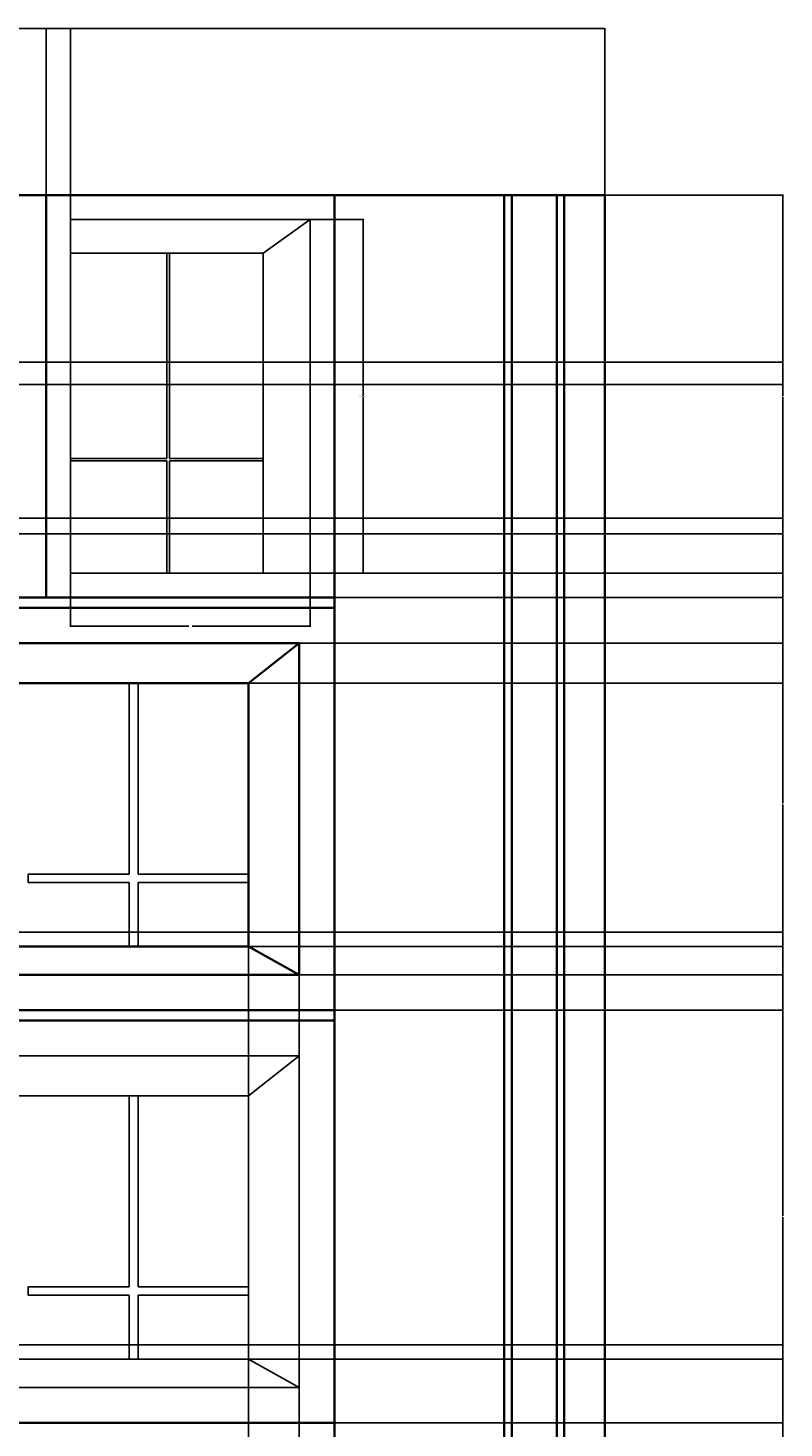
# Model space of a CAD drawing. Units: feet. Extents: x 1141 to 2858, y 751 to 1654.
# Tile 13 of 13: x 2610 to 2858, y 1195 to 1654. Entities that reach past the tile are written whole.
import ezdxf

# ---------------------------------------------------------------- set-up
doc = ezdxf.new("R2010")
doc.units = ezdxf.units.FT
for name, color, linetype, lineweight in [('A-ANNO-DIMS', 2, 'Continuous', 18), ('A-ELEV', 7, 'Continuous', 35), ('A-GLAZ', 4, 'Continuous', 25)]:
    doc.layers.add(name, color=color, linetype=linetype, lineweight=lineweight)
doc.styles.get("Standard").update_dxf_attribs({"font": 'arial.ttf'})
doc.dimstyles.get("Standard").update_dxf_attribs({"dimtxt": 0.18, "dimasz": 0.18, "dimexe": 0.18, "dimexo": 0.0625, "dimgap": 0.09, "dimtad": 0, "dimtih": 1, "dimtoh": 1, "dimdec": 1, "dimzin": 0, "dimdsep": 46, "dimlunit": 3, "dimtxsty": 'Standard', "dimcen": 0.09, "dimadec": 0, "dimazin": 0, "dimtfac": 1, "dimtdec": 1, "dimtofl": 0, "dimtmove": 0, "dimatfit": 3, "dimfxl": 1, "dimtolj": 1, "dimtzin": 0, "dimarcsym": 0})

# ---------------------------------------------------------------- blocks, each defined once
blk = doc.blocks.new('WIN-SIDE-B')
blk.add_line((63.09, 104.94), (78.57, 116.03))
blk.add_lwpolyline([(78.57, 0), (0, 0), (0, 116.03), (78.57, 116.03)], close=True)
for points in [[(63.09, 0), (63.09, 104.94), (0, 104.94)], [(31.54, 37.61), (31.54, 104.94), (32.46, 104.94), (32.46, 37.61)], [(31.54, 36.79), (0, 36.79), (0, 37.61), (31.54, 37.61)], [(32.46, 36.79), (32.46, 0), (31.54, 0), (31.54, 36.79)], [(32.46, 37.61), (63.09, 37.61), (63.09, 36.79), (32.46, 36.79)]]:
    blk.add_lwpolyline(points)
blk = doc.blocks.new('BALCONY-GLAZ-B')
for p, q in [((0, 108.84), (16.63, 95.74)), ((266.62, 95.74), (273.67, 108.84)), ((16.63, 95.74), (16.63, 9.29)), ((16.63, 95.74), (266.62, 95.74)), ((266.62, 95.74), (266.62, 9.19)), ((16.63, 9.29), (0, 0)), ((16.63, 9.29), (266.62, 9.29)), ((266.62, 9.29), (273.67, 0))]:
    blk.add_line(p, q)
for points in [[(0, 108.84), (273.67, 108.84), (273.67, 0), (0, 0)], [(266.62, 9.19), (168.47, 9.19), (168.47, 95.74), (266.62, 95.74)]]:
    blk.add_lwpolyline(points, close=True)
blk = doc.blocks.new('WIN-SLIDING')
for points in [[(36.16, 23.71), (36.16, 86.44), (39.2, 86.44), (39.2, 23.71)], [(36.16, 23.71), (0, 23.71), (0, 21.05), (36.16, 21.05)], [(39.2, 21.05), (72.32, 21.05), (72.32, 23.71), (39.2, 23.71)], [(39.2, 21.05), (39.2, 0), (36.16, 0), (36.16, 21.05)]]:
    blk.add_lwpolyline(points)
blk = doc.blocks.new('*D16')
at = {"layer": 'A-ANNO-DIMS', "color": 0, "lineweight": -2, "transparency": 16777216}
for p, q in [((2702.75, 1591.47), (2720.27, 1591.47)), ((2720.09, 1591.29), (2720.09, 1533.64)), ((2720.09, 1475.62), (2720.09, 1533.27)), ((2702.75, 1475.44), (2720.27, 1475.44))]:
    blk.add_line(p, q, dxfattribs=at)
at = {"layer": 'A-ANNO-DIMS', "color": 0, "transparency": 16777216}
for points in [[(2720.06, 1591.29), (2720.12, 1591.29), (2720.09, 1591.47)], [(2720.06, 1475.62), (2720.12, 1475.62), (2720.09, 1475.44)]]:
    blk.add_solid(points, dxfattribs=at)
at = {"layer": 'Defpoints', "color": 0, "transparency": 16777216}
for p in [(2702.69, 1591.47), (2720.09, 1591.47), (2702.69, 1475.44)]:
    blk.add_point(p, dxfattribs=at)
at = {"layer": 'A-ANNO-DIMS', "color": 0, "transparency": 16777216, "insert": (2720.09, 1533.45), "char_height": 0.18, "attachment_point": 5}
blk.add_mtext('\\A1;SIDE WINDOW B 116 TYP.', dxfattribs=at)
blk = doc.blocks.new('*D17')
at = {"layer": 'A-ANNO-DIMS', "color": 0, "lineweight": -2, "transparency": 16777216}
for p, q in [((2624.12, 1475.38), (2624.12, 1457.85)), ((2702.69, 1475.38), (2702.69, 1457.85)), ((2624.3, 1458.03), (2662.88, 1458.03)), ((2702.51, 1458.03), (2663.93, 1458.03))]:
    blk.add_line(p, q, dxfattribs=at)
at = {"layer": 'A-ANNO-DIMS', "color": 0, "transparency": 16777216}
for points in [[(2624.3, 1458.06), (2624.3, 1458), (2624.12, 1458.03)], [(2702.51, 1458.06), (2702.51, 1458), (2702.69, 1458.03)]]:
    blk.add_solid(points, dxfattribs=at)
at = {"layer": 'Defpoints', "color": 0, "transparency": 16777216}
for p in [(2624.12, 1475.44), (2702.69, 1475.44), (2702.69, 1458.03)]:
    blk.add_point(p, dxfattribs=at)
at = {"layer": 'A-ANNO-DIMS', "color": 0, "transparency": 16777216, "insert": (2663.41, 1458.03), "char_height": 0.18, "attachment_point": 5}
blk.add_mtext('\\A1;79 TYP.', dxfattribs=at)
blk = doc.blocks.new('*D31')
at = {"layer": 'A-ANNO-DIMS', "color": 0, "lineweight": -2, "transparency": 16777216}
for p, q in [((2117.47, 1196.68), (2857.83, 1196.68)), ((2857.65, 1196.5), (2857.65, 1129.16)), ((2857.65, 1061.47), (2857.65, 1128.8)), ((2117.47, 1061.29), (2857.83, 1061.29))]:
    blk.add_line(p, q, dxfattribs=at)
at = {"layer": 'A-ANNO-DIMS', "color": 0, "transparency": 16777216}
for points in [[(2857.62, 1196.5), (2857.68, 1196.5), (2857.65, 1196.68)], [(2857.62, 1061.47), (2857.68, 1061.47), (2857.65, 1061.29)]]:
    blk.add_solid(points, dxfattribs=at)
at = {"layer": 'Defpoints', "color": 0, "transparency": 16777216}
for p in [(2117.41, 1196.68), (2857.65, 1196.68), (2117.41, 1061.29)]:
    blk.add_point(p, dxfattribs=at)
at = {"layer": 'A-ANNO-DIMS', "color": 0, "transparency": 16777216, "insert": (2857.65, 1128.98), "char_height": 0.18, "attachment_point": 5}
blk.add_mtext('\\A1;135.4', dxfattribs=at)
blk = doc.blocks.new('*D32')
at = {"layer": 'A-ANNO-DIMS', "color": 0, "lineweight": -2, "transparency": 16777216}
for p, q in [((2117.47, 1332.06), (2857.83, 1332.06)), ((2857.65, 1331.88), (2857.65, 1264.55)), ((2857.65, 1196.86), (2857.65, 1264.19)), ((2117.47, 1196.68), (2857.83, 1196.68))]:
    blk.add_line(p, q, dxfattribs=at)
at = {"layer": 'A-ANNO-DIMS', "color": 0, "transparency": 16777216}
for points in [[(2857.62, 1331.88), (2857.68, 1331.88), (2857.65, 1332.06)], [(2857.62, 1196.86), (2857.68, 1196.86), (2857.65, 1196.68)]]:
    blk.add_solid(points, dxfattribs=at)
at = {"layer": 'Defpoints', "color": 0, "transparency": 16777216}
for p in [(2117.41, 1332.06), (2857.65, 1332.06), (2117.41, 1196.68)]:
    blk.add_point(p, dxfattribs=at)
at = {"layer": 'A-ANNO-DIMS', "color": 0, "transparency": 16777216, "insert": (2857.65, 1264.37), "char_height": 0.18, "attachment_point": 5}
blk.add_mtext('\\A1;135.4', dxfattribs=at)
blk = doc.blocks.new('*D33')
at = {"layer": 'A-ANNO-DIMS', "color": 0, "lineweight": -2, "transparency": 16777216}
for p, q in [((2117.47, 1467.45), (2857.83, 1467.45)), ((2857.65, 1467.27), (2857.65, 1399.94)), ((2857.65, 1332.24), (2857.65, 1399.58)), ((2117.47, 1332.06), (2857.83, 1332.06))]:
    blk.add_line(p, q, dxfattribs=at)
at = {"layer": 'A-ANNO-DIMS', "color": 0, "transparency": 16777216}
for points in [[(2857.62, 1467.27), (2857.68, 1467.27), (2857.65, 1467.45)], [(2857.62, 1332.24), (2857.68, 1332.24), (2857.65, 1332.06)]]:
    blk.add_solid(points, dxfattribs=at)
at = {"layer": 'Defpoints', "color": 0, "transparency": 16777216}
for p in [(2117.41, 1467.45), (2857.65, 1467.45), (2117.41, 1332.06)]:
    blk.add_point(p, dxfattribs=at)
at = {"layer": 'A-ANNO-DIMS', "color": 0, "transparency": 16777216, "insert": (2857.65, 1399.76), "char_height": 0.18, "attachment_point": 5}
blk.add_mtext('\\A1;135.4', dxfattribs=at)
blk = doc.blocks.new('*D34')
at = {"layer": 'A-ANNO-DIMS', "color": 0, "lineweight": -2, "transparency": 16777216}
for p, q in [((2117.47, 1599.45), (2857.83, 1599.45)), ((2857.65, 1599.27), (2857.65, 1533.63)), ((2857.65, 1467.63), (2857.65, 1533.27)), ((2117.47, 1467.45), (2857.83, 1467.45))]:
    blk.add_line(p, q, dxfattribs=at)
at = {"layer": 'A-ANNO-DIMS', "color": 0, "transparency": 16777216}
for points in [[(2857.62, 1599.27), (2857.68, 1599.27), (2857.65, 1599.45)], [(2857.62, 1467.63), (2857.68, 1467.63), (2857.65, 1467.45)]]:
    blk.add_solid(points, dxfattribs=at)
at = {"layer": 'Defpoints', "color": 0, "transparency": 16777216}
for p in [(2117.41, 1599.45), (2857.65, 1599.45), (2117.41, 1467.45)]:
    blk.add_point(p, dxfattribs=at)
at = {"layer": 'A-ANNO-DIMS', "color": 0, "transparency": 16777216, "insert": (2857.65, 1533.45), "char_height": 0.18, "attachment_point": 5}
blk.add_mtext('\\A1;132', dxfattribs=at)
blk = doc.blocks.new('*D35')
at = {"layer": 'A-ANNO-DIMS', "color": 0, "lineweight": -2, "transparency": 16777216}
for p, q in [((2319.3, 1599.52), (2319.3, 1654.28)), ((2319.48, 1654.1), (2559.01, 1654.1)), ((2799.12, 1654.1), (2559.59, 1654.1)), ((2799.3, 1599.52), (2799.3, 1654.28))]:
    blk.add_line(p, q, dxfattribs=at)
at = {"layer": 'A-ANNO-DIMS', "color": 0, "transparency": 16777216}
for points in [[(2319.48, 1654.13), (2319.48, 1654.07), (2319.3, 1654.1)], [(2799.12, 1654.13), (2799.12, 1654.07), (2799.3, 1654.1)]]:
    blk.add_solid(points, dxfattribs=at)
at = {"layer": 'Defpoints', "color": 0, "transparency": 16777216}
for p in [(2799.3, 1654.1), (2319.3, 1599.45), (2799.3, 1599.45)]:
    blk.add_point(p, dxfattribs=at)
at = {"layer": 'A-ANNO-DIMS', "color": 0, "transparency": 16777216, "insert": (2559.3, 1654.1), "char_height": 0.18, "attachment_point": 5}
blk.add_mtext('\\A1;480', dxfattribs=at)
blk = doc.blocks.new('*D46')
at = {"layer": 'A-ANNO-DIMS', "color": 0, "lineweight": -2, "transparency": 16777216}
for p, q in [((2604.56, 1587.93), (2604.56, 1654.28)), ((2604.74, 1654.1), (2609.96, 1654.1)), ((2615.96, 1654.1), (2610.73, 1654.1)), ((2616.14, 1599.52), (2616.14, 1654.28))]:
    blk.add_line(p, q, dxfattribs=at)
at = {"layer": 'A-ANNO-DIMS', "color": 0, "transparency": 16777216}
for points in [[(2604.74, 1654.13), (2604.74, 1654.07), (2604.56, 1654.1)], [(2615.96, 1654.13), (2615.96, 1654.07), (2616.14, 1654.1)]]:
    blk.add_solid(points, dxfattribs=at)
at = {"layer": 'Defpoints', "color": 0, "transparency": 16777216}
for p in [(2616.14, 1654.1), (2616.14, 1599.45), (2604.56, 1587.87)]:
    blk.add_point(p, dxfattribs=at)
at = {"layer": 'A-ANNO-DIMS', "color": 0, "transparency": 16777216, "insert": (2610.35, 1654.1), "char_height": 0.18, "attachment_point": 5}
blk.add_mtext('\\A1;11.58', dxfattribs=at)
blk = doc.blocks.new('*D47')
at = {"layer": 'A-ANNO-DIMS', "color": 0, "lineweight": -2, "transparency": 16777216}
for p, q in [((2616.14, 1599.52), (2616.14, 1654.28)), ((2616.32, 1654.1), (2619.74, 1654.1)), ((2623.94, 1654.1), (2620.52, 1654.1)), ((2624.12, 1591.53), (2624.12, 1654.28))]:
    blk.add_line(p, q, dxfattribs=at)
at = {"layer": 'A-ANNO-DIMS', "color": 0, "transparency": 16777216}
for points in [[(2616.32, 1654.13), (2616.32, 1654.07), (2616.14, 1654.1)], [(2623.94, 1654.13), (2623.94, 1654.07), (2624.12, 1654.1)]]:
    blk.add_solid(points, dxfattribs=at)
at = {"layer": 'Defpoints', "color": 0, "transparency": 16777216}
for p in [(2624.12, 1654.1), (2616.14, 1599.45), (2624.12, 1591.47)]:
    blk.add_point(p, dxfattribs=at)
at = {"layer": 'A-ANNO-DIMS', "color": 0, "transparency": 16777216, "insert": (2620.13, 1654.1), "char_height": 0.18, "attachment_point": 5}
blk.add_mtext('\\A1;7.986', dxfattribs=at)
blk = doc.blocks.new('*D64')
at = {"layer": 'A-ANNO-DIMS', "color": 0, "lineweight": -2, "transparency": 16777216}
for p, q in [((2507.45, 1544.65), (2857.83, 1544.65)), ((2857.65, 1544.47), (2857.65, 1541.17)), ((2857.65, 1537.51), (2857.65, 1540.81)), ((2507.45, 1537.33), (2857.83, 1537.33))]:
    blk.add_line(p, q, dxfattribs=at)
at = {"layer": 'A-ANNO-DIMS', "color": 0, "transparency": 16777216}
for points in [[(2857.62, 1544.47), (2857.68, 1544.47), (2857.65, 1544.65)], [(2857.62, 1537.51), (2857.68, 1537.51), (2857.65, 1537.33)]]:
    blk.add_solid(points, dxfattribs=at)
at = {"layer": 'Defpoints', "color": 0, "transparency": 16777216}
for p in [(2507.39, 1544.65), (2507.39, 1537.33), (2857.65, 1537.33)]:
    blk.add_point(p, dxfattribs=at)
at = {"layer": 'A-ANNO-DIMS', "color": 0, "transparency": 16777216, "insert": (2857.65, 1540.99), "char_height": 0.18, "attachment_point": 5}
blk.add_mtext('\\A1;7.317', dxfattribs=at)
blk = doc.blocks.new('*D65')
at = {"layer": 'A-ANNO-DIMS', "color": 0, "lineweight": -2, "transparency": 16777216}
for p, q in [((2507.45, 1493.43), (2857.83, 1493.43)), ((2857.65, 1493.25), (2857.65, 1491.06)), ((2507.45, 1488.33), (2857.83, 1488.33)), ((2857.65, 1488.51), (2857.65, 1490.69))]:
    blk.add_line(p, q, dxfattribs=at)
at = {"layer": 'A-ANNO-DIMS', "color": 0, "transparency": 16777216}
for points in [[(2857.62, 1493.25), (2857.68, 1493.25), (2857.65, 1493.43)], [(2857.62, 1488.51), (2857.68, 1488.51), (2857.65, 1488.33)]]:
    blk.add_solid(points, dxfattribs=at)
at = {"layer": 'Defpoints', "color": 0, "transparency": 16777216}
for p in [(2507.39, 1493.43), (2507.39, 1488.33), (2857.65, 1488.33)]:
    blk.add_point(p, dxfattribs=at)
at = {"layer": 'A-ANNO-DIMS', "color": 0, "transparency": 16777216, "insert": (2857.65, 1490.88), "char_height": 0.18, "attachment_point": 5}
blk.add_mtext('\\A1;5.099', dxfattribs=at)
blk = doc.blocks.new('*D66')
at = {"layer": 'A-ANNO-DIMS', "color": 0, "lineweight": -2, "transparency": 16777216}
for p, q in [((2702.75, 1475.44), (2857.83, 1475.44)), ((2857.65, 1475.26), (2857.65, 1471.63)), ((2857.65, 1467.63), (2857.65, 1471.26)), ((2710.74, 1467.45), (2857.83, 1467.45))]:
    blk.add_line(p, q, dxfattribs=at)
at = {"layer": 'A-ANNO-DIMS', "color": 0, "transparency": 16777216}
for points in [[(2857.62, 1475.26), (2857.68, 1475.26), (2857.65, 1475.44)], [(2857.62, 1467.63), (2857.68, 1467.63), (2857.65, 1467.45)]]:
    blk.add_solid(points, dxfattribs=at)
at = {"layer": 'Defpoints', "color": 0, "transparency": 16777216}
for p in [(2702.69, 1475.44), (2857.65, 1475.44), (2710.68, 1467.45)]:
    blk.add_point(p, dxfattribs=at)
at = {"layer": 'A-ANNO-DIMS', "color": 0, "transparency": 16777216, "insert": (2857.65, 1471.45), "char_height": 0.18, "attachment_point": 5}
blk.add_mtext('\\A1;7.986', dxfattribs=at)
blk = doc.blocks.new('*D71')
at = {"layer": 'A-ANNO-DIMS', "color": 0, "lineweight": -2, "transparency": 16777216}
for p, q in [((2682.47, 1352.88), (2682.47, 751.07)), ((2699.1, 1343.58), (2699.1, 751.07)), ((2682.65, 751.25), (2690.4, 751.25)), ((2698.92, 751.25), (2691.17, 751.25))]:
    blk.add_line(p, q, dxfattribs=at)
at = {"layer": 'A-ANNO-DIMS', "color": 0, "transparency": 16777216}
for points in [[(2682.65, 751.28), (2682.65, 751.22), (2682.47, 751.25)], [(2698.92, 751.28), (2698.92, 751.22), (2699.1, 751.25)]]:
    blk.add_solid(points, dxfattribs=at)
at = {"layer": 'Defpoints', "color": 0, "transparency": 16777216}
for p in [(2682.47, 1352.94), (2699.1, 1343.65), (2699.1, 751.25)]:
    blk.add_point(p, dxfattribs=at)
at = {"layer": 'A-ANNO-DIMS', "color": 0, "transparency": 16777216, "insert": (2690.78, 751.25), "char_height": 0.18, "attachment_point": 5}
blk.add_mtext('\\A1;16.63', dxfattribs=at)
blk = doc.blocks.new('*D72')
at = {"layer": 'A-ANNO-DIMS', "color": 0, "lineweight": -2, "transparency": 16777216}
for p, q in [((2699.1, 1343.58), (2699.1, 751.07)), ((2710.68, 1332), (2710.68, 751.07)), ((2699.28, 751.25), (2704.5, 751.25)), ((2710.5, 751.25), (2705.27, 751.25))]:
    blk.add_line(p, q, dxfattribs=at)
at = {"layer": 'A-ANNO-DIMS', "color": 0, "transparency": 16777216}
for points in [[(2699.28, 751.28), (2699.28, 751.22), (2699.1, 751.25)], [(2710.5, 751.28), (2710.5, 751.22), (2710.68, 751.25)]]:
    blk.add_solid(points, dxfattribs=at)
at = {"layer": 'Defpoints', "color": 0, "transparency": 16777216}
for p in [(2699.1, 1343.65), (2710.68, 1332.06), (2710.68, 751.25)]:
    blk.add_point(p, dxfattribs=at)
at = {"layer": 'A-ANNO-DIMS', "color": 0, "transparency": 16777216, "insert": (2704.89, 751.25), "char_height": 0.18, "attachment_point": 5}
blk.add_mtext('\\A1;11.58', dxfattribs=at)
blk = doc.blocks.new('*D74')
at = {"layer": 'A-ANNO-DIMS', "color": 0, "lineweight": -2, "transparency": 16777216}
for p, q in [((2413.84, 1332), (2413.84, 751.07)), ((2710.68, 1332), (2710.68, 751.07)), ((2414.02, 751.25), (2561.79, 751.25)), ((2710.5, 751.25), (2562.72, 751.25))]:
    blk.add_line(p, q, dxfattribs=at)
at = {"layer": 'A-ANNO-DIMS', "color": 0, "transparency": 16777216}
for points in [[(2414.02, 751.28), (2414.02, 751.22), (2413.84, 751.25)], [(2710.5, 751.28), (2710.5, 751.22), (2710.68, 751.25)]]:
    blk.add_solid(points, dxfattribs=at)
at = {"layer": 'Defpoints', "color": 0, "transparency": 16777216}
for p in [(2413.84, 1332.06), (2710.68, 1332.06), (2710.68, 751.25)]:
    blk.add_point(p, dxfattribs=at)
at = {"layer": 'A-ANNO-DIMS', "color": 0, "transparency": 16777216, "insert": (2562.26, 751.25), "char_height": 0.18, "attachment_point": 5}
blk.add_mtext('\\A1;296.83', dxfattribs=at)
blk = doc.blocks.new('*D75')
at = {"layer": 'A-ANNO-DIMS', "color": 0, "lineweight": -2, "transparency": 16777216}
for p, q in [((2699.16, 1343.65), (2857.83, 1343.65)), ((2857.65, 1343.47), (2857.65, 1338.04)), ((2857.65, 1332.24), (2857.65, 1337.67)), ((2710.74, 1332.06), (2857.83, 1332.06))]:
    blk.add_line(p, q, dxfattribs=at)
at = {"layer": 'A-ANNO-DIMS', "color": 0, "transparency": 16777216}
for points in [[(2857.62, 1343.47), (2857.68, 1343.47), (2857.65, 1343.65)], [(2857.62, 1332.24), (2857.68, 1332.24), (2857.65, 1332.06)]]:
    blk.add_solid(points, dxfattribs=at)
at = {"layer": 'Defpoints', "color": 0, "transparency": 16777216}
for p in [(2699.1, 1343.65), (2857.65, 1343.65), (2710.68, 1332.06)]:
    blk.add_point(p, dxfattribs=at)
at = {"layer": 'A-ANNO-DIMS', "color": 0, "transparency": 16777216, "insert": (2857.65, 1337.85), "char_height": 0.18, "attachment_point": 5}
blk.add_mtext('\\A1;11.58', dxfattribs=at)
blk = doc.blocks.new('*D76')
at = {"layer": 'A-ANNO-DIMS', "color": 0, "lineweight": -2, "transparency": 16777216}
for p, q in [((2682.53, 1352.94), (2857.83, 1352.94)), ((2857.65, 1352.76), (2857.65, 1348.47)), ((2857.65, 1343.83), (2857.65, 1348.11)), ((2699.16, 1343.65), (2857.83, 1343.65))]:
    blk.add_line(p, q, dxfattribs=at)
at = {"layer": 'A-ANNO-DIMS', "color": 0, "transparency": 16777216}
for points in [[(2857.62, 1352.76), (2857.68, 1352.76), (2857.65, 1352.94)], [(2857.62, 1343.83), (2857.68, 1343.83), (2857.65, 1343.65)]]:
    blk.add_solid(points, dxfattribs=at)
at = {"layer": 'Defpoints', "color": 0, "transparency": 16777216}
for p in [(2682.47, 1352.94), (2857.65, 1352.94), (2699.1, 1343.65)]:
    blk.add_point(p, dxfattribs=at)
at = {"layer": 'A-ANNO-DIMS', "color": 0, "transparency": 16777216, "insert": (2857.65, 1348.29), "char_height": 0.18, "attachment_point": 5}
blk.add_mtext('\\A1;9.293', dxfattribs=at)
blk = doc.blocks.new('*D77')
at = {"layer": 'A-ANNO-DIMS', "color": 0, "lineweight": -2, "transparency": 16777216}
for p, q in [((2699.16, 1452.48), (2857.83, 1452.48)), ((2857.65, 1452.3), (2857.65, 1446.12)), ((2857.65, 1439.56), (2857.65, 1445.75)), ((2682.53, 1439.38), (2857.83, 1439.38))]:
    blk.add_line(p, q, dxfattribs=at)
at = {"layer": 'A-ANNO-DIMS', "color": 0, "transparency": 16777216}
for points in [[(2857.62, 1452.3), (2857.68, 1452.3), (2857.65, 1452.48)], [(2857.62, 1439.56), (2857.68, 1439.56), (2857.65, 1439.38)]]:
    blk.add_solid(points, dxfattribs=at)
at = {"layer": 'Defpoints', "color": 0, "transparency": 16777216}
for p in [(2699.1, 1452.48), (2857.65, 1452.48), (2682.47, 1439.38)]:
    blk.add_point(p, dxfattribs=at)
at = {"layer": 'A-ANNO-DIMS', "color": 0, "transparency": 16777216, "insert": (2857.65, 1445.93), "char_height": 0.18, "attachment_point": 5}
blk.add_mtext('\\A1;13.102', dxfattribs=at)
blk = doc.blocks.new('*D84')
at = {"layer": 'A-ANNO-DIMS', "color": 0, "lineweight": -2, "transparency": 16777216}
for p, q in [((2458.84, 1222.24), (2857.83, 1222.24)), ((2857.65, 1222.06), (2857.65, 1209.64)), ((2857.65, 1196.86), (2857.65, 1209.27)), ((2319.36, 1196.68), (2857.83, 1196.68))]:
    blk.add_line(p, q, dxfattribs=at)
at = {"layer": 'A-ANNO-DIMS', "color": 0, "transparency": 16777216}
for points in [[(2857.62, 1222.06), (2857.68, 1222.06), (2857.65, 1222.24)], [(2857.62, 1196.86), (2857.68, 1196.86), (2857.65, 1196.68)]]:
    blk.add_solid(points, dxfattribs=at)
at = {"layer": 'Defpoints', "color": 0, "transparency": 16777216}
for p in [(2458.78, 1222.24), (2857.65, 1222.24), (2319.3, 1196.68)]:
    blk.add_point(p, dxfattribs=at)
at = {"layer": 'A-ANNO-DIMS', "color": 0, "transparency": 16777216, "insert": (2857.65, 1209.46), "char_height": 0.18, "attachment_point": 5}
blk.add_mtext('\\A1;25.56', dxfattribs=at)
blk = doc.blocks.new('*D85')
at = {"layer": 'A-ANNO-DIMS', "color": 0, "lineweight": -2, "transparency": 16777216}
for p, q in [((2610.2, 1217.55), (2857.83, 1217.55)), ((2857.65, 1217.37), (2857.65, 1207.3)), ((2857.65, 1196.86), (2857.65, 1206.93)), ((2319.36, 1196.68), (2857.83, 1196.68))]:
    blk.add_line(p, q, dxfattribs=at)
at = {"layer": 'A-ANNO-DIMS', "color": 0, "transparency": 16777216}
for points in [[(2857.62, 1217.37), (2857.68, 1217.37), (2857.65, 1217.55)], [(2857.62, 1196.86), (2857.68, 1196.86), (2857.65, 1196.68)]]:
    blk.add_solid(points, dxfattribs=at)
at = {"layer": 'Defpoints', "color": 0, "transparency": 16777216}
for p in [(2610.14, 1217.55), (2857.65, 1217.55), (2319.3, 1196.68)]:
    blk.add_point(p, dxfattribs=at)
at = {"layer": 'A-ANNO-DIMS', "color": 0, "transparency": 16777216, "insert": (2857.65, 1207.11), "char_height": 0.18, "attachment_point": 5}
blk.add_mtext('\\A1;20.873', dxfattribs=at)
blk = doc.blocks.new('*D87')
at = {"layer": 'A-ANNO-DIMS', "color": 0, "lineweight": -2, "transparency": 16777216}
for p, q in [((2458.84, 1357.62), (2857.83, 1357.62)), ((2857.65, 1357.44), (2857.65, 1345.03)), ((2857.65, 1332.24), (2857.65, 1344.66)), ((2413.9, 1332.06), (2857.83, 1332.06))]:
    blk.add_line(p, q, dxfattribs=at)
at = {"layer": 'A-ANNO-DIMS', "color": 0, "transparency": 16777216}
for points in [[(2857.62, 1357.44), (2857.68, 1357.44), (2857.65, 1357.62)], [(2857.62, 1332.24), (2857.68, 1332.24), (2857.65, 1332.06)]]:
    blk.add_solid(points, dxfattribs=at)
at = {"layer": 'Defpoints', "color": 0, "transparency": 16777216}
for p in [(2458.78, 1357.62), (2857.65, 1357.62), (2413.84, 1332.06)]:
    blk.add_point(p, dxfattribs=at)
at = {"layer": 'A-ANNO-DIMS', "color": 0, "transparency": 16777216, "insert": (2857.65, 1344.84), "char_height": 0.18, "attachment_point": 5}
blk.add_mtext('\\A1;25.56', dxfattribs=at)
blk = doc.blocks.new('*D88')
at = {"layer": 'A-ANNO-DIMS', "color": 0, "lineweight": -2, "transparency": 16777216}
for p, q in [((2682.53, 1352.94), (2857.83, 1352.94)), ((2857.65, 1352.76), (2857.65, 1342.68)), ((2857.65, 1332.24), (2857.65, 1342.32)), ((2413.9, 1332.06), (2857.83, 1332.06))]:
    blk.add_line(p, q, dxfattribs=at)
at = {"layer": 'A-ANNO-DIMS', "color": 0, "transparency": 16777216}
for points in [[(2857.62, 1352.76), (2857.68, 1352.76), (2857.65, 1352.94)], [(2857.62, 1332.24), (2857.68, 1332.24), (2857.65, 1332.06)]]:
    blk.add_solid(points, dxfattribs=at)
at = {"layer": 'Defpoints', "color": 0, "transparency": 16777216}
for p in [(2682.47, 1352.94), (2857.65, 1352.94), (2413.84, 1332.06)]:
    blk.add_point(p, dxfattribs=at)
at = {"layer": 'A-ANNO-DIMS', "color": 0, "transparency": 16777216, "insert": (2857.65, 1342.5), "char_height": 0.18, "attachment_point": 5}
blk.add_mtext('\\A1;20.873', dxfattribs=at)

msp = doc.modelspace()

# ---------------------------------------------------------------- linework, layer by layer
at = {"layer": 'A-ELEV'}
for p, q in [((2699.0959, 1452.4845), (2682.4659, 1439.3822)), ((2682.4659, 1439.3822), (2432.4759, 1439.3822)), ((2682.4659, 1439.3822), (2682.4659, 1352.9376)), ((2682.4659, 1352.9376), (2432.4759, 1352.9376)), ((2682.4659, 1352.9376), (2699.0959, 1343.645))]:
    msp.add_line(p, q, dxfattribs=at)
for points in [[(2319.3013, 1599.4527), (2616.1358, 1599.4527), (2616.1358, 1467.4527), (2319.3013, 1467.4527)], [(2710.6762, 1467.4527), (2616.1358, 1467.4527), (2616.1358, 1599.4527), (2710.6762, 1599.4527)], [(2710.6762, 1464.0647), (2413.8417, 1464.0647), (2413.8417, 1332.0647), (2710.6762, 1332.0647)], [(2699.0959, 1452.4845), (2425.4219, 1452.4845), (2425.4219, 1343.645), (2699.0959, 1343.645)], [(2710.6762, 1328.6768), (2413.8417, 1328.6768), (2413.8417, 1196.6768), (2710.6762, 1196.6768)]]:
    msp.add_lwpolyline(points, close=True, dxfattribs=at)
for points in [[(2799.3013, 919.339), (2799.3013, 1599.4527), (2710.6762, 1599.4527), (2710.6762, 919.339)], [(2768.7322, 919.339), (2768.7322, 1599.4527), (2766.2848, 1599.4527), (2766.2848, 919.339)], [(2785.9583, 919.339), (2785.9583, 1599.4527), (2783.5108, 1599.4527), (2783.5108, 919.339)]]:
    msp.add_lwpolyline(points, dxfattribs=at)

# ---------------------------------------------------------------- block references
at = {"layer": 'A-GLAZ'}
msp.add_blockref('WIN-SIDE-B', (2624.122, 1475.439), dxfattribs=at)
at = {"layer": 'A-GLAZ', "extrusion": (0, 0, -1), "zscale": -1}
for name, p in [('WIN-SLIDING', (-2682.4662, 1352.9379)), ('BALCONY-GLAZ-B', (-2699.0954, 1208.257)), ('WIN-SLIDING', (-2682.4662, 1217.55))]:
    msp.add_blockref(name, p, dxfattribs=at)

# ---------------------------------------------------------------- dimensions: what is measured, and where the dimension line sits
at = {"layer": 'A-ANNO-DIMS'}
for base, p1, p2, override, picture, middle in [((2799.3013, 1654.1027), (2319.3013, 1599.4527), (2799.3013, 1599.4527), {"dimdec": 0, "dimlfac": 1, "dimrnd": 0, "dimzin": 0, "dimdsep": 46, "dimlunit": 2}, '*D35', (2559.3013, 1654.1027)), ((2616.1358, 1654.1027), (2604.5555, 1587.8725), (2616.1358, 1599.4527), {"dimdec": 2, "dimlfac": 1, "dimrnd": 0, "dimzin": 0, "dimdsep": 46, "dimlunit": 2}, '*D46', (2610.3457, 1654.1027)), ((2624.1217, 1654.1027), (2616.1358, 1599.4527), (2624.1217, 1591.4669), {"dimdec": 3, "dimlfac": 1, "dimrnd": 0, "dimzin": 0, "dimdsep": 46, "dimlunit": 2}, '*D47', (2620.1287, 1654.1027)), ((2699.0959, 751.2508), (2682.4659, 1352.9376), (2699.0959, 1343.645), {"dimdec": 2, "dimlfac": 1, "dimrnd": 0, "dimzin": 0, "dimdsep": 46, "dimlunit": 2}, '*D71', (2690.7809, 751.2508)), ((2710.6762, 751.2508), (2699.0959, 1343.645), (2710.6762, 1332.0647), {"dimdec": 2, "dimlfac": 1, "dimrnd": 0, "dimzin": 0, "dimdsep": 46, "dimlunit": 2}, '*D72', (2704.886, 751.2508)), ((2710.6762, 751.2508), (2413.8417, 1332.0647), (2710.6762, 1332.0647), {"dimdec": 2, "dimlfac": 1, "dimrnd": 0, "dimzin": 0, "dimdsep": 46, "dimlunit": 2}, '*D74', (2562.2589, 751.2508))]:
    dim = msp.add_linear_dim(base=base, p1=p1, p2=p2, dimstyle='Standard', override=override, dxfattribs=at)
    dim.commit()
    dim.dimension.update_dxf_attribs({"geometry": picture, "text_midpoint": middle})
for base, p1, p2, override, picture, middle in [((2857.6489, 1599.4527), (2117.407, 1467.4527), (2117.407, 1599.4527), {"dimdec": 0, "dimlfac": 1, "dimrnd": 0, "dimzin": 0, "dimdsep": 46, "dimlunit": 2}, '*D34', (2857.6489, 1533.4527)), ((2857.6489, 1537.3285), (2507.3869, 1544.6458), (2507.3869, 1537.3285), {"dimdec": 3, "dimlfac": 1, "dimrnd": 0, "dimzin": 0, "dimdsep": 46, "dimlunit": 2}, '*D64', (2857.6489, 1540.9872)), ((2857.64893, 1488.32554), (2507.38694, 1493.42501), (2507.38694, 1488.32554), {"dimdec": 3, "dimlfac": 1, "dimrnd": 0, "dimzin": 0, "dimdsep": 46, "dimlunit": 2}, '*D65', (2857.64893, 1490.87527)), ((2857.6489, 1475.4386), (2710.6762, 1467.4527), (2702.6903, 1475.4386), {"dimdec": 3, "dimlfac": 1, "dimrnd": 0, "dimzin": 0, "dimdsep": 46, "dimlunit": 2}, '*D66', (2857.6489, 1471.4457)), ((2857.6489, 1467.4527), (2117.407, 1332.0647), (2117.407, 1467.4527), {"dimdec": 1, "dimlfac": 1, "dimrnd": 0, "dimzin": 0, "dimdsep": 46, "dimlunit": 2}, '*D33', (2857.6489, 1399.7587)), ((2857.6489, 1452.4845), (2682.4659, 1439.3822), (2699.0959, 1452.4845), {"dimdec": 3, "dimlfac": 1, "dimrnd": 0, "dimzin": 0, "dimdsep": 46, "dimlunit": 2}, '*D77', (2857.6489, 1445.9334)), ((2857.6489, 1357.6233), (2413.8417, 1332.0647), (2458.7755, 1357.6233), {"dimdec": 2, "dimlfac": 1, "dimrnd": 0, "dimzin": 0, "dimdsep": 46, "dimlunit": 2}, '*D87', (2857.6489, 1344.844)), ((2857.6489, 1352.9376), (2413.8417, 1332.0647), (2682.4659, 1352.9376), {"dimdec": 3, "dimlfac": 1, "dimrnd": 0, "dimzin": 0, "dimdsep": 46, "dimlunit": 2}, '*D88', (2857.6489, 1342.5012)), ((2857.6489, 1352.9376), (2699.0959, 1343.645), (2682.4659, 1352.9376), {"dimdec": 3, "dimlfac": 1, "dimrnd": 0, "dimzin": 0, "dimdsep": 46, "dimlunit": 2}, '*D76', (2857.6489, 1348.2913)), ((2857.6489, 1343.645), (2710.6762, 1332.0647), (2699.0959, 1343.645), {"dimdec": 2, "dimlfac": 1, "dimrnd": 0, "dimzin": 0, "dimdsep": 46, "dimlunit": 2}, '*D75', (2857.6489, 1337.8549)), ((2857.6489, 1332.0647), (2117.407, 1196.6768), (2117.407, 1332.0647), {"dimdec": 1, "dimlfac": 1, "dimrnd": 0, "dimzin": 0, "dimdsep": 46, "dimlunit": 2}, '*D32', (2857.6489, 1264.3708)), ((2857.6489, 1222.2353), (2319.3013, 1196.6768), (2458.7755, 1222.2353), {"dimdec": 2, "dimlfac": 1, "dimrnd": 0, "dimzin": 0, "dimdsep": 46, "dimlunit": 2}, '*D84', (2857.6489, 1209.456)), ((2857.6489, 1217.5496), (2319.3013, 1196.6768), (2610.1419, 1217.5496), {"dimdec": 3, "dimlfac": 1, "dimrnd": 0, "dimzin": 0, "dimdsep": 46, "dimlunit": 2}, '*D85', (2857.6489, 1207.1132)), ((2857.6489, 1196.6768), (2117.407, 1061.2888), (2117.407, 1196.6768), {"dimdec": 1, "dimlfac": 1, "dimrnd": 0, "dimzin": 0, "dimdsep": 46, "dimlunit": 2}, '*D31', (2857.6489, 1128.9828))]:
    dim = msp.add_linear_dim(base=base, p1=p1, p2=p2, angle=90, dimstyle='Standard', override=override, dxfattribs=at)
    dim.commit()
    dim.dimension.update_dxf_attribs({"geometry": picture, "text_midpoint": middle})
dim = msp.add_linear_dim(base=(2720.0945, 1591.4669), p1=(2702.6903, 1475.4386), p2=(2702.6903, 1591.4669), angle=90, text='SIDE WINDOW B <> TYP.', dimstyle='Standard', override={"dimdec": 0, "dimlfac": 1, "dimrnd": 0, "dimzin": 0, "dimdsep": 46, "dimlunit": 2}, dxfattribs=at)
dim.commit()
dim.dimension.update_dxf_attribs({"geometry": '*D16', "text_midpoint": (2720.0945, 1533.4527)})
dim = msp.add_linear_dim(base=(2702.6903, 1458.0344), p1=(2624.1217, 1475.4386), p2=(2702.6903, 1475.4386), text='<> TYP.', dimstyle='Standard', override={"dimdec": 0, "dimlfac": 1, "dimrnd": 0, "dimzin": 0, "dimdsep": 46, "dimlunit": 2}, dxfattribs=at)
dim.commit()
dim.dimension.update_dxf_attribs({"geometry": '*D17', "text_midpoint": (2663.406, 1458.0344)})

doc.saveas('drawing.dxf')
